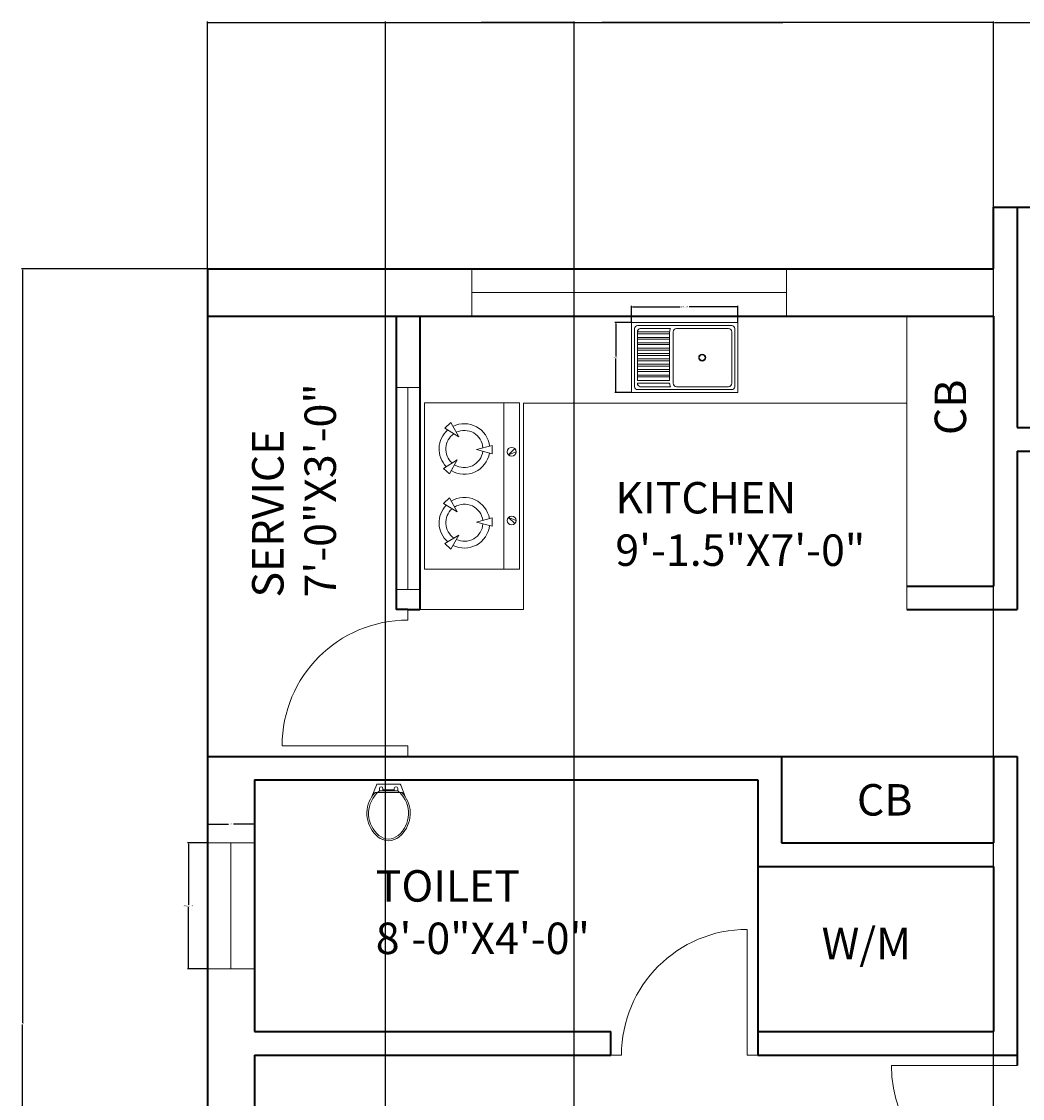
# Model space of a CAD drawing. Units: inches. Extents: x -59 to 444, y -680 to 63.
# Tile 5 of 9: x -59 to 132, y -143 to 63. Entities that reach past the tile are written whole.
import ezdxf

# ---------------------------------------------------------------- set-up
doc = ezdxf.new("R2010")
doc.units = ezdxf.units.IN
doc.header["$MEASUREMENT"] = 0
for name, color, linetype, lineweight in [('A-ANNO-DIMS', 2, 'Continuous', 18), ('A-ANNO-TEXT', 7, 'Continuous', 18), ('A-AREA-IDEN', 7, 'Continuous', 18), ('A-DOOR', 3, 'Continuous', 18), ('A-EQPM', 9, 'Continuous', 18), ('A-FLOR-CASE', 8, 'Continuous', 18), ('A-FLOR-FIXT', 9, 'Continuous', 18), ('A-GLAZ', 4, 'Continuous', 18), ('A-WALL', 7, 'Continuous', 35)]:
    doc.layers.add(name, color=color, linetype=linetype, lineweight=lineweight)
doc.styles.get("Standard").update_dxf_attribs({"font": 'arial.ttf'})
doc.dimstyles.get("Standard").update_dxf_attribs({"dimtxt": 0.18, "dimasz": 0.18, "dimexe": 0.18, "dimexo": 0.0625, "dimgap": 0.09, "dimtad": 0, "dimtih": 1, "dimtoh": 1, "dimdec": 0, "dimzin": 0, "dimdsep": 46, "dimlunit": 3, "dimtxsty": 'Standard', "dimcen": 0.09, "dimadec": 0, "dimazin": 0, "dimtfac": 1, "dimtdec": 0, "dimtofl": 0, "dimtmove": 0, "dimatfit": 3, "dimfxl": 1, "dimtolj": 1, "dimtzin": 0, "dimarcsym": 0})

# ---------------------------------------------------------------- blocks, each defined once
blk = doc.blocks.new('М12 540х820')
for p, q in [((0, 540), (-820, 540)), ((-820, 540), (-820, 0)), ((-45, 517.5), (-775, 517.5)), ((0, 0), (0, 540)), ((-797.5, 495), (-797.5, 45)), ((-775, 468), (-775, 72)), ((-347.5, 495), (-748, 495)), ((-320.5, 468), (-320.5, 72)), ((-301.7, 495), (-64.8, 495)), ((-293.7, 468), (-293.7, 472.5)), ((-293.7, 468), (-45, 468)), ((-293.7, 446.6), (-45, 446.6)), ((-293.7, 419.6), (-293.7, 446.6)), ((-293.7, 419.6), (-45, 419.6)), ((-45, 469.5), (-45, 468)), ((-45, 419.6), (-45, 446.6)), ((-22.5, 45), (-22.5, 495)), ((-293.7, 405), (-45, 405)), ((-293.7, 378), (-293.7, 405)), ((-293.7, 378), (-45, 378)), ((-293.7, 336.4), (-293.7, 363.4)), ((-293.7, 363.4), (-45, 363.4)), ((-293.7, 336.4), (-45, 336.4)), ((-45, 378), (-45, 405)), ((-45, 336.4), (-45, 363.4)), ((-293.7, 294.7), (-293.7, 321.7)), ((-293.7, 321.7), (-45, 321.7)), ((-293.7, 294.7), (-45, 294.7)), ((-293.7, 253.1), (-293.7, 280.1)), ((-293.7, 280.1), (-45, 280.1)), ((-293.7, 253.1), (-45, 253.1)), ((-45, 294.7), (-45, 321.7)), ((-45, 253.1), (-45, 280.1)), ((-293.7, 211.5), (-293.7, 238.5)), ((-293.7, 238.5), (-45, 238.5)), ((-293.7, 211.5), (-45, 211.5)), ((-293.7, 169.9), (-293.7, 196.9)), ((-293.7, 196.9), (-45, 196.9)), ((-293.7, 169.9), (-45, 169.9)), ((-45, 211.5), (-45, 238.5)), ((-45, 169.9), (-45, 196.9)), ((-293.7, 128.2), (-293.7, 155.2)), ((-293.7, 155.2), (-45, 155.2)), ((-293.7, 128.2), (-45, 128.2)), ((-293.7, 113.6), (-45, 113.6)), ((-293.7, 86.6), (-293.7, 113.6)), ((-293.7, 86.6), (-45, 86.6)), ((-45, 128.2), (-45, 155.2)), ((-45, 86.6), (-45, 113.6)), ((-820, 0), (0, 0)), ((-775, 22.5), (-45, 22.5)), ((-748, 45), (-347.5, 45)), ((-301.7, 45), (-64.8, 45)), ((-293.7, 72), (-45, 72)), ((-45, 70.5), (-45, 72))]:
    blk.add_line(p, q)
at = {"ltscale": 0.06}
for p, q in [((-820, 0), (-820, 540)), ((-820, 540), (0, 540)), ((0, 540), (0, 536.9)), ((0, 536.9), (0, 0)), ((-293.7, 446.6), (-45, 446.6)), ((-293.7, 405), (-293.7, 446.6)), ((-45, 446.6), (-45, 419.6)), ((-45, 419.6), (-45, 378)), ((-293.7, 363.4), (-293.7, 405)), ((-293.7, 321.7), (-293.7, 363.4)), ((-45, 378), (-45, 336.4)), ((-45, 336.4), (-45, 294.7)), ((-293.7, 280.1), (-293.7, 321.7)), ((-293.7, 238.5), (-293.7, 280.1)), ((-45, 294.7), (-45, 253.1)), ((-45, 253.1), (-45, 211.5)), ((-293.7, 196.9), (-293.7, 238.5)), ((-293.7, 155.2), (-293.7, 196.9)), ((-45, 211.5), (-45, 169.9)), ((-45, 169.9), (-45, 128.2)), ((-293.7, 113.6), (-293.7, 155.2)), ((-293.7, 72), (-293.7, 113.6)), ((-45, 128.2), (-45, 86.6)), ((-45, 86.6), (-45, 72)), ((0, 0), (-820, 0)), ((-45, 72), (-293.7, 72))]:
    blk.add_line(p, q, dxfattribs=at)
at = {"extrusion": (0, 0, -1)}
for centre, major_axis, start_param, end_param in [((-775, 495), (-15.9, 15.9), -0.785398, 0.785398), ((-775, 495), (-15.9, 15.9), -0.785398, 0.785398), ((-45, 495), (-15.9, -15.9), 2.356194, 3.926991), ((-45, 495), (-15.9, -15.9), 2.356194, 3.926991), ((-748, 468), (-19.1, -19.1), 0.785398, 2.356194), ((-748, 468), (-19.1, -19.1), 0.785398, 2.356194), ((-347.5, 468), (-19.1, 19.1), 0.785398, 2.356194), ((-347.5, 468), (-19.1, 19.1), 0.785398, 2.356194), ((-343.2, 468), (-35, 35), 1.779263, 2.356194), ((-343.2, 468), (-35, 35), 1.779263, 2.356192), ((-343.2, 468), (-35, 35), 2.356192, 2.356194), ((-72.3, 468.8), (-19.3, 19.3), 1.0328, 2.38382), ((-72.3, 468.8), (-19.3, 19.3), 1.0328, 1.064673), ((-72.3, 468.8), (-19.3, 19.3), 1.064673, 2.328569), ((-72.3, 468.8), (-19.3, 19.3), 2.328569, 2.38382), ((-545.5, 270), (-19.1, -19.1), 3.926991, 10.210176), ((-545.5, 270), (-19.1, -19.1), 3.926991, 10.210176), ((-545.5, 270), (-15.9, -15.9), 3.926991, 10.210176), ((-545.5, 270), (-15.9, -15.9), 3.926991, 10.210176), ((-775, 45), (-15.9, -15.9), 5.497787, 7.068583), ((-775, 45), (-15.9, -15.9), 5.497787, 7.068583), ((-748, 72), (-19.1, 19.1), 3.926991, 5.497787), ((-748, 72), (-19.1, 19.1), 3.926991, 5.497787), ((-347.5, 72), (-19.1, -19.1), 3.926991, 5.497787), ((-347.5, 72), (-19.1, -19.1), 3.926991, 5.497787), ((-343.2, 72), (-35, -35), 3.926991, 4.503922), ((-343.2, 72), (-35, -35), 3.926991, 4.503922), ((-72.3, 71.2), (-19.3, -19.3), 3.899365, 5.250385), ((-72.3, 71.2), (-19.3, -19.3), 5.218512, 5.250385), ((-72.3, 71.2), (-19.3, -19.3), 3.954617, 5.218512), ((-72.3, 71.2), (-19.3, -19.3), 3.899365, 3.954617), ((-45, 45), (-15.9, 15.9), 2.356194, 3.926991), ((-45, 45), (-15.9, 15.9), 2.356194, 3.926991)]:
    blk.add_ellipse(centre, major_axis=major_axis, ratio=1, start_param=start_param, end_param=end_param, dxfattribs=at)
blk = doc.blocks.new('WC-COMPACT')
for p, q in [((1.55, 9.19), (2, 9.19)), ((2, 9.19), (4.13, 9.19)), ((6.26, 9.19), (4.13, 9.19)), ((6.26, 9.19), (6.72, 9.19))]:
    blk.add_line(p, q)
for points in [[(4.13, 10.83), (2.07, 10.83, 0.31031), (1.81, 10.65), (0.96, 8.45, 0.209071)], [(2.38, 9.52), (2.38, 9.97, -1), (3.07, 9.97), (3.07, 9.73)], [(4.13, 10.83), (6.2, 10.83, -0.31031), (6.46, 10.65), (7.3, 8.45, -0.209071)], [(5.89, 9.52), (5.89, 9.97, 1), (5.2, 9.97), (5.2, 9.73)], [(0.96, 8.45, 0.383919), (2.1, 0.78, 0.163732), (4.13, 0, 0.359733)], [(1.79, 8.97, 0.431639), (2.3, 1.03, 0.162618), (4.13, 0.32, 0.470877)], [(1.55, 9.19, 0.040937), (0.96, 8.45, 0.163732)], [(2, 9.19, 0.014165), (1.79, 8.97, 0.162618)], [(2.38, 9.52, 0.022712), (2, 9.19, 0.162618)], [(4.13, 9.52), (2.38, 9.52, 0.022712)], [(4.13, 9.52), (5.89, 9.52, -0.476108)], [(6.26, 9.19, -0.448546), (5.96, 1.03, -0.162618), (4.13, 0.32, -0.470877)], [(7.3, 8.45, -0.383919), (6.17, 0.78, -0.163732), (4.13, 0, -0.359733)], [(5.89, 9.52, -0.022712), (6.26, 9.19, -0.162618)], [(6.72, 9.19, -0.040937), (7.3, 8.45, -0.163732)]]:
    blk.add_lwpolyline(points, format="xyb")
for points in [[(5.2, 9.73), (3.07, 9.73)], [(3.07, 9.73), (3.07, 9.52)], [(5.2, 9.73), (5.2, 9.52)]]:
    blk.add_lwpolyline(points)
blk = doc.blocks.new('WIN-60-W9')
for p, q in [((60, 9), (0, 9)), ((0, 9), (0, 0)), ((60, 0), (60, 9)), ((0, 4.5), (60, 4.5)), ((0, 0), (60, 0))]:
    blk.add_line(p, q)
blk = doc.blocks.new('WIN-24-W9')
for p, q in [((0, 24), (0, 0)), ((9, 24), (0, 24)), ((4.5, 24), (4.5, 0)), ((9, 0), (9, 24)), ((0, 0), (9, 0))]:
    blk.add_line(p, q)
blk = doc.blocks.new('WIN-SERVICE')
for p, q in [((0, 38.53), (0, 0)), ((4.5, 38.53), (0, 38.53)), ((2.25, 38.53), (2.25, 0)), ((4.5, 38.53), (4.5, 0)), ((0, 0), (4.5, 0))]:
    blk.add_line(p, q)
blk = doc.blocks.new('DOOR-SWING-24')
blk.add_line((24, 0), (0, 0))
blk.add_arc((24, 0), 24, 90, 180)
blk = doc.blocks.new('*D22')
at = {"layer": 'A-ANNO-DIMS', "color": 0, "lineweight": -2, "transparency": 16777216}
for p, q in [((-23.33, -93.94), (-27.05, -93.94)), ((-26.87, -94.12), (-26.87, -105.75)), ((-26.87, -117.76), (-26.87, -106.12)), ((-23.33, -117.94), (-27.05, -117.94))]:
    blk.add_line(p, q, dxfattribs=at)
at = {"layer": 'A-ANNO-DIMS', "color": 0, "transparency": 16777216}
for points in [[(-26.9, -94.12), (-26.84, -94.12), (-26.87, -93.94)], [(-26.9, -117.76), (-26.84, -117.76), (-26.87, -117.94)]]:
    blk.add_solid(points, dxfattribs=at)
at = {"layer": 'Defpoints', "color": 0, "transparency": 16777216}
for p in [(-23.27, -93.94), (-26.87, -117.94), (-23.27, -117.94)]:
    blk.add_point(p, dxfattribs=at)
at = {"layer": 'A-ANNO-DIMS', "color": 0, "transparency": 16777216, "insert": (-26.87, -105.94), "char_height": 0.18, "attachment_point": 5}
blk.add_mtext('\\A1;WINDOW 24 TYP.', dxfattribs=at)
blk = doc.blocks.new('*D23')
at = {"layer": 'A-ANNO-DIMS', "color": 0, "lineweight": -2, "transparency": 16777216}
for p, q in [((-23.27, -93.87), (-23.27, -90.16)), ((-23.09, -90.34), (-19.23, -90.34)), ((-14.45, -90.34), (-18.31, -90.34)), ((-14.27, -93.87), (-14.27, -90.16))]:
    blk.add_line(p, q, dxfattribs=at)
at = {"layer": 'A-ANNO-DIMS', "color": 0, "transparency": 16777216}
for points in [[(-23.09, -90.31), (-23.09, -90.37), (-23.27, -90.34)], [(-14.45, -90.31), (-14.45, -90.37), (-14.27, -90.34)]]:
    blk.add_solid(points, dxfattribs=at)
at = {"layer": 'Defpoints', "color": 0, "transparency": 16777216}
for p in [(-23.27, -90.34), (-23.27, -93.94), (-14.27, -93.94)]:
    blk.add_point(p, dxfattribs=at)
at = {"layer": 'A-ANNO-DIMS', "color": 0, "transparency": 16777216, "insert": (-18.77, -90.34), "char_height": 0.18, "attachment_point": 5}
blk.add_mtext('\\A1;9 TYP.', dxfattribs=at)
blk = doc.blocks.new('*D28')
at = {"layer": 'A-ANNO-DIMS', "color": 0, "lineweight": -2, "transparency": 16777216}
for p, q in [((57.67, 5.36), (57.67, 8.51)), ((57.85, 8.33), (66.93, 8.33)), ((77.72, 8.33), (68.64, 8.33)), ((77.9, 5.36), (77.9, 8.51))]:
    blk.add_line(p, q, dxfattribs=at)
at = {"layer": 'A-ANNO-DIMS', "color": 0, "transparency": 16777216}
for points in [[(57.85, 8.36), (57.85, 8.3), (57.67, 8.33)], [(77.72, 8.36), (77.72, 8.3), (77.9, 8.33)]]:
    blk.add_solid(points, dxfattribs=at)
at = {"layer": 'Defpoints', "color": 0, "transparency": 16777216}
for p in [(57.67, 8.33), (57.67, 5.3), (77.9, 5.3)]:
    blk.add_point(p, dxfattribs=at)
at = {"layer": 'A-ANNO-DIMS', "color": 0, "transparency": 16777216, "insert": (67.79, 8.33), "char_height": 0.18, "attachment_point": 5}
blk.add_mtext('\\A1;SINK 20 TYP.', dxfattribs=at)
blk = doc.blocks.new('*D29')
at = {"layer": 'A-ANNO-DIMS', "color": 0, "lineweight": -2, "transparency": 16777216}
for p, q in [((57.61, 5.3), (54.46, 5.3)), ((54.64, 5.12), (54.64, -1.18)), ((54.64, -7.84), (54.64, -1.54)), ((57.61, -8.02), (54.46, -8.02))]:
    blk.add_line(p, q, dxfattribs=at)
at = {"layer": 'A-ANNO-DIMS', "color": 0, "transparency": 16777216}
for points in [[(54.61, 5.12), (54.67, 5.12), (54.64, 5.3)], [(54.61, -7.84), (54.67, -7.84), (54.64, -8.02)]]:
    blk.add_solid(points, dxfattribs=at)
at = {"layer": 'Defpoints', "color": 0, "transparency": 16777216}
for p in [(57.67, 5.3), (54.64, -8.02), (57.67, -8.02)]:
    blk.add_point(p, dxfattribs=at)
at = {"layer": 'A-ANNO-DIMS', "color": 0, "transparency": 16777216, "insert": (54.64, -1.36), "char_height": 0.18, "attachment_point": 5}
blk.add_mtext('\\A1;13 TYP.', dxfattribs=at)
blk = doc.blocks.new('*D48')
at = {"layer": 'A-ANNO-DIMS', "color": 0, "lineweight": -2, "transparency": 16777216}
for p, q in [((-23.33, 15.56), (-58.7, 15.56)), ((-58.52, 15.38), (-58.52, -128.25)), ((-58.52, -272.26), (-58.52, -128.62)), ((-23.33, -272.44), (-58.7, -272.44))]:
    blk.add_line(p, q, dxfattribs=at)
at = {"layer": 'A-ANNO-DIMS', "color": 0, "transparency": 16777216}
for points in [[(-58.55, 15.38), (-58.49, 15.38), (-58.52, 15.56)], [(-58.55, -272.26), (-58.49, -272.26), (-58.52, -272.44)]]:
    blk.add_solid(points, dxfattribs=at)
at = {"layer": 'Defpoints', "color": 0, "transparency": 16777216}
for p in [(-23.27, 15.56), (-58.52, -272.44), (-23.27, -272.44)]:
    blk.add_point(p, dxfattribs=at)
at = {"layer": 'A-ANNO-DIMS', "color": 0, "transparency": 16777216, "insert": (-58.52, -128.44), "char_height": 0.18, "attachment_point": 5}
blk.add_mtext('\\A1;288', dxfattribs=at)
blk = doc.blocks.new('*D51')
at = {"layer": 'A-ANNO-DIMS', "color": 0, "lineweight": -2, "transparency": 16777216}
for p, q in [((-23.27, 15.63), (-23.27, 62.74)), ((-23.09, 62.56), (51.45, 62.56)), ((126.55, 62.56), (52.01, 62.56)), ((126.73, 27.38), (126.73, 62.74))]:
    blk.add_line(p, q, dxfattribs=at)
at = {"layer": 'A-ANNO-DIMS', "color": 0, "transparency": 16777216}
for points in [[(-23.09, 62.59), (-23.09, 62.53), (-23.27, 62.56)], [(126.55, 62.59), (126.55, 62.53), (126.73, 62.56)]]:
    blk.add_solid(points, dxfattribs=at)
at = {"layer": 'Defpoints', "color": 0, "transparency": 16777216}
for p in [(126.73, 62.56), (126.73, 27.31), (-23.27, 15.56)]:
    blk.add_point(p, dxfattribs=at)
at = {"layer": 'A-ANNO-DIMS', "color": 0, "transparency": 16777216, "insert": (51.73, 62.56), "char_height": 0.18, "attachment_point": 5}
blk.add_mtext('\\A1;150', dxfattribs=at)
blk = doc.blocks.new('*D52')
at = {"layer": 'A-ANNO-DIMS', "color": 0, "lineweight": -2, "transparency": 16777216}
for p, q in [((126.73, 27.38), (126.73, 62.74)), ((126.91, 62.56), (196.97, 62.56)), ((267.55, 62.56), (197.49, 62.56)), ((267.73, 27.38), (267.73, 62.74))]:
    blk.add_line(p, q, dxfattribs=at)
at = {"layer": 'A-ANNO-DIMS', "color": 0, "transparency": 16777216}
for points in [[(126.91, 62.59), (126.91, 62.53), (126.73, 62.56)], [(267.55, 62.59), (267.55, 62.53), (267.73, 62.56)]]:
    blk.add_solid(points, dxfattribs=at)
at = {"layer": 'Defpoints', "color": 0, "transparency": 16777216}
for p in [(267.73, 62.56), (126.73, 27.31), (267.73, 27.31)]:
    blk.add_point(p, dxfattribs=at)
at = {"layer": 'A-ANNO-DIMS', "color": 0, "transparency": 16777216, "insert": (197.23, 62.56), "char_height": 0.18, "attachment_point": 5}
blk.add_mtext('\\A1;141', dxfattribs=at)
blk = doc.blocks.new('*D54')
at = {"layer": 'A-ANNO-DIMS', "color": 0, "lineweight": -2, "transparency": 16777216}
for p, q in [((10.73, -344.37), (10.73, 62.74)), ((10.91, 62.56), (28.51, 62.56)), ((46.55, 62.56), (28.95, 62.56)), ((46.73, -344.37), (46.73, 62.74))]:
    blk.add_line(p, q, dxfattribs=at)
at = {"layer": 'A-ANNO-DIMS', "color": 0, "transparency": 16777216}
for points in [[(10.91, 62.59), (10.91, 62.53), (10.73, 62.56)], [(46.55, 62.59), (46.55, 62.53), (46.73, 62.56)]]:
    blk.add_solid(points, dxfattribs=at)
at = {"layer": 'Defpoints', "color": 0, "transparency": 16777216}
for p in [(46.73, 62.56), (10.73, -344.44), (46.73, -344.44)]:
    blk.add_point(p, dxfattribs=at)
at = {"layer": 'A-ANNO-DIMS', "color": 0, "transparency": 16777216, "insert": (28.73, 62.56), "char_height": 0.18, "attachment_point": 5}
blk.add_mtext('\\A1;36', dxfattribs=at)
blk = doc.blocks.new('*D55')
at = {"layer": 'A-ANNO-DIMS', "color": 0, "lineweight": -2, "transparency": 16777216}
for p, q in [((46.73, -344.37), (46.73, 62.74)), ((46.91, 62.56), (86.51, 62.56)), ((126.55, 62.56), (86.95, 62.56)), ((126.73, -344.37), (126.73, 62.74))]:
    blk.add_line(p, q, dxfattribs=at)
at = {"layer": 'A-ANNO-DIMS', "color": 0, "transparency": 16777216}
for points in [[(46.91, 62.59), (46.91, 62.53), (46.73, 62.56)], [(126.55, 62.59), (126.55, 62.53), (126.73, 62.56)]]:
    blk.add_solid(points, dxfattribs=at)
at = {"layer": 'Defpoints', "color": 0, "transparency": 16777216}
for p in [(126.73, 62.56), (46.73, -344.44), (126.73, -344.44)]:
    blk.add_point(p, dxfattribs=at)
at = {"layer": 'A-ANNO-DIMS', "color": 0, "transparency": 16777216, "insert": (86.73, 62.56), "char_height": 0.18, "attachment_point": 5}
blk.add_mtext('\\A1;80', dxfattribs=at)
blk = doc.blocks.new('*D56')
at = {"layer": 'A-ANNO-DIMS', "color": 0, "lineweight": -2, "transparency": 16777216}
for p, q in [((126.73, -344.37), (126.73, 62.74)), ((126.91, 62.56), (158.65, 62.56)), ((191.05, 62.56), (159.3, 62.56)), ((191.23, -344.37), (191.23, 62.74))]:
    blk.add_line(p, q, dxfattribs=at)
at = {"layer": 'A-ANNO-DIMS', "color": 0, "transparency": 16777216}
for points in [[(126.91, 62.59), (126.91, 62.53), (126.73, 62.56)], [(191.05, 62.59), (191.05, 62.53), (191.23, 62.56)]]:
    blk.add_solid(points, dxfattribs=at)
at = {"layer": 'Defpoints', "color": 0, "transparency": 16777216}
for p in [(191.23, 62.56), (126.73, -344.44), (191.23, -344.44)]:
    blk.add_point(p, dxfattribs=at)
at = {"layer": 'A-ANNO-DIMS', "color": 0, "transparency": 16777216, "insert": (158.98, 62.56), "char_height": 0.18, "attachment_point": 5}
blk.add_mtext('\\A1;64.5', dxfattribs=at)

msp = doc.modelspace()

# ---------------------------------------------------------------- linework, layer by layer
at = {"layer": 'A-DOOR'}
for p, q in [((14.98, -51.44), (14.98, -49.44)), ((14.98, -77.44), (14.98, -75.44)), ((55.73, -134.44), (53.73, -134.44)), ((81.73, -134.44), (79.73, -134.44)), ((131.23, -136.44), (107.23, -136.44))]:
    msp.add_line(p, q, dxfattribs=at)
msp.add_arc((131.75, -136.44), 24.52, 180, 258.1877, dxfattribs=at)
at = {"layer": 'A-EQPM'}
for p, q in [((33.31, -10.02), (33.31, -41.73)), ((22.06, -14.85), (23.18, -13.75)), ((23.18, -13.75), (24.68, -16.45)), ((24.68, -16.45), (22.06, -14.85)), ((28.05, -18.89), (31.03, -18.15)), ((31.03, -18.15), (31.03, -19.71)), ((31.03, -19.71), (28.05, -18.89)), ((21.77, -22.49), (24.4, -20.86)), ((22.92, -23.56), (21.77, -22.49)), ((24.4, -20.86), (22.92, -23.56)), ((22.92, -28.12), (21.77, -29.18)), ((24.4, -30.81), (22.92, -28.12)), ((21.77, -29.18), (24.4, -30.81)), ((31.03, -31.96), (28.05, -32.78)), ((28.05, -32.78), (31.03, -33.53)), ((31.03, -33.53), (31.03, -31.96)), ((24.68, -35.22), (22.06, -36.82)), ((22.06, -36.82), (23.18, -37.92)), ((23.18, -37.92), (24.68, -35.22))]:
    msp.add_line(p, q, dxfattribs=at)
at = {"layer": 'A-EQPM', "ltscale": 20}
for p, q in [((34.2, -19.92), (35.37, -18.73)), ((35.62, -19.32), (34.2, -19.92)), ((34.2, -31.84), (35.37, -33.02)), ((35.62, -32.43), (34.2, -31.84))]:
    msp.add_line(p, q, dxfattribs=at)
at = {"layer": 'A-EQPM'}
msp.add_lwpolyline([(18.13, -41.73), (18.13, -10.02), (36.25, -10.02), (36.25, -41.73)], close=True, dxfattribs=at)
at = {"layer": 'A-EQPM', "ltscale": 20}
for centre in [(34.78, -19.32), (34.78, -32.43)]:
    msp.add_circle(centre, 0.834, dxfattribs=at)
at = {"layer": 'A-EQPM'}
for centre, radius, start, end in [((25.76, -18.8), 4.83, 6.4005, 116.769), ((25.76, -18.8), 4.83, 131.2225, 224.1627), ((25.76, -18.8), 3.54, 124.5561, 228.8027), ((25.76, -18.8), 3.54, 3.5753, 115.9207), ((25.76, -18.8), 4.83, 238.853, 350.7562), ((25.76, -18.8), 3.54, 237.9778, 353.02), ((25.76, -32.87), 4.83, 9.2438, 121.147), ((25.76, -32.87), 4.83, 135.8373, 228.7775), ((25.76, -32.87), 3.54, 131.1973, 235.4439), ((25.76, -32.87), 3.54, 6.98, 122.0222), ((25.76, -32.87), 4.83, 243.231, 353.5995), ((25.76, -32.87), 3.54, 244.0793, 356.4247)]:
    msp.add_arc(centre, radius, start, end, dxfattribs=at)
at = {"layer": 'A-FLOR-CASE'}
for p, q in [((110.14, -49.44), (110.14, 6.56)), ((37.06, -49.44), (37.06, -10.04)), ((37.06, -10.04), (110.14, -10.04)), ((17.23, -49.44), (37.06, -49.44))]:
    msp.add_line(p, q, dxfattribs=at)
at = {"layer": 'A-WALL'}
for p, q in [((126.73, 15.56), (126.73, 27.31)), ((126.73, 27.31), (131.23, 27.31)), ((131.23, 27.31), (131.23, -14.69)), ((131.23, 27.31), (263.23, 27.31)), ((-23.27, 15.56), (126.73, 15.56)), ((-23.27, 15.56), (-23.27, -272.44)), ((-23.27, 6.56), (126.73, 6.56)), ((12.73, 6.56), (12.73, -49.44)), ((17.23, 6.56), (17.23, -49.44)), ((126.73, 6.56), (126.73, -44.94)), ((131.23, -14.69), (173.23, -14.69)), ((131.23, -19.19), (173.23, -19.19)), ((131.23, -19.19), (131.23, -49.44)), ((110.14, -44.94), (126.73, -44.94)), ((14.98, -49.44), (12.73, -49.44)), ((14.98, -49.44), (17.23, -49.44)), ((110.14, -49.44), (131.23, -49.44)), ((-23.27, -77.44), (131.23, -77.44)), ((12.73, -77.44), (17.23, -77.44)), ((86.23, -77.44), (86.23, -93.94)), ((126.73, -77.44), (126.73, -93.94)), ((131.23, -77.44), (131.23, -136.44)), ((-14.27, -81.94), (81.73, -81.94)), ((-14.27, -81.94), (-14.27, -129.94)), ((81.73, -81.94), (81.73, -134.44)), ((86.23, -93.94), (126.73, -93.94)), ((81.73, -98.44), (126.73, -98.44)), ((126.73, -98.44), (126.73, -129.94)), ((-14.27, -129.94), (53.73, -129.94)), ((53.73, -134.44), (53.73, -129.94)), ((81.73, -129.94), (126.73, -129.94)), ((-14.27, -134.44), (53.73, -134.44)), ((-14.27, -134.44), (-14.27, -263.44)), ((81.73, -134.44), (131.23, -134.44))]:
    msp.add_line(p, q, dxfattribs=at)

# ---------------------------------------------------------------- block references
at = {"layer": 'A-DOOR'}
msp.add_blockref('DOOR-SWING-24', (-9.02, -75.44), dxfattribs=at)
at = {"layer": 'A-DOOR', "extrusion": (0, 0, -1), "zscale": -1, "rotation": 270}
msp.add_blockref('DOOR-SWING-24', (-79.73, -110.44), dxfattribs=at)
at = {"layer": 'A-FLOR-FIXT', "xscale": 0.0246684035300764, "yscale": 0.0246684035300764, "zscale": 0.0246684035300764, "rotation": 180}
msp.add_blockref('М12 540х820', (57.67, 5.3), dxfattribs=at)
at = {"layer": 'A-FLOR-FIXT'}
msp.add_blockref('WC-COMPACT', (7.16, -93.55), dxfattribs=at)
at = {"layer": 'A-GLAZ'}
for name, p in [('WIN-60-W9', (27.19, 6.56)), ('WIN-SERVICE', (12.73, -45.59))]:
    msp.add_blockref(name, p, dxfattribs=at)
at = {"layer": 'A-GLAZ', "rotation": 180}
msp.add_blockref('WIN-24-W9', (-14.27, -93.94), dxfattribs=at)

# ---------------------------------------------------------------- texts
at = {"layer": 'A-ANNO-TEXT', "insert": (115.48, -16.14), "char_height": 6, "attachment_point": 1, "rotation": 90}
msp.add_mtext('CB', dxfattribs=at)
at = {"layer": 'A-ANNO-TEXT', "char_height": 6, "attachment_point": 1}
for s, insert in [('CB', (100.65, -82.73)), ('W/M', (93.92, -110.14))]:
    msp.add_mtext(s, dxfattribs=dict(at, insert=insert))
at = {"layer": 'A-AREA-IDEN', "insert": (-14.74, -47.13), "char_height": 6, "attachment_point": 1, "rotation": 90}
msp.add_mtext('SERVICE\\P7\'-0"X3\'-0"', dxfattribs=at)
at = {"layer": 'A-AREA-IDEN', "char_height": 6, "attachment_point": 1}
for s, insert in [('KITCHEN\\P9\'-1.5"X7\'-0"', (54.56, -25.1)), ('TOILET\\P8\'-0"X4\'-0"', (8.85, -99.15))]:
    msp.add_mtext(s, dxfattribs=dict(at, insert=insert))

# ---------------------------------------------------------------- dimensions: what is measured, and where the dimension line sits
at = {"layer": 'A-ANNO-DIMS'}
for base, p1, p2, override, picture, middle in [((126.73, 62.56), (-23.27, 15.56), (126.73, 27.31), {"dimdec": 0, "dimlfac": 1, "dimrnd": 0, "dimzin": 0, "dimdsep": 46, "dimlunit": 2}, '*D51', (51.73, 62.56)), ((46.73, 62.56), (10.73, -344.44), (46.73, -344.44), {"dimdec": 0, "dimlfac": 1, "dimrnd": 0, "dimzin": 0, "dimdsep": 46, "dimlunit": 2}, '*D54', (28.73, 62.56)), ((126.73, 62.56), (46.73, -344.44), (126.73, -344.44), {"dimdec": 0, "dimlfac": 1, "dimrnd": 0, "dimzin": 0, "dimdsep": 46, "dimlunit": 2}, '*D55', (86.73, 62.56)), ((267.73, 62.56), (126.73, 27.31), (267.73, 27.31), {"dimdec": 0, "dimlfac": 1, "dimrnd": 0, "dimzin": 0, "dimdsep": 46, "dimlunit": 2}, '*D52', (197.23, 62.56)), ((191.23, 62.56), (126.73, -344.44), (191.23, -344.44), {"dimdec": 1, "dimlfac": 1, "dimrnd": 0, "dimzin": 0, "dimdsep": 46, "dimlunit": 2}, '*D56', (158.98, 62.56))]:
    dim = msp.add_linear_dim(base=base, p1=p1, p2=p2, dimstyle='Standard', override=override, dxfattribs=at)
    dim.commit()
    dim.dimension.update_dxf_attribs({"geometry": picture, "text_midpoint": middle})
dim = msp.add_linear_dim(base=(-58.52, -272.44), p1=(-23.27, 15.56), p2=(-23.27, -272.44), angle=90, dimstyle='Standard', override={"dimdec": 0, "dimlfac": 1, "dimrnd": 0, "dimzin": 0, "dimdsep": 46, "dimlunit": 2}, dxfattribs=at)
dim.commit()
dim.dimension.update_dxf_attribs({"geometry": '*D48', "text_midpoint": (-58.52, -128.44)})
for base, p1, p2, angle, text, picture, middle in [((57.67, 8.33), (77.9, 5.3), (57.67, 5.3), 180, 'SINK <> TYP.', '*D28', (67.79, 8.33)), ((54.64, -8.02), (57.67, 5.3), (57.67, -8.02), 270, '<> TYP.', '*D29', (54.64, -1.36)), ((-23.27, -90.34), (-14.27, -93.94), (-23.27, -93.94), 180, '<> TYP.', '*D23', (-18.77, -90.34)), ((-26.87, -117.94), (-23.27, -93.94), (-23.27, -117.94), 270, 'WINDOW <> TYP.', '*D22', (-26.87, -105.94))]:
    dim = msp.add_linear_dim(base=base, p1=p1, p2=p2, angle=angle, text=text, dimstyle='Standard', override={"dimdec": 0, "dimlfac": 1, "dimrnd": 0, "dimzin": 0, "dimdsep": 46, "dimlunit": 2}, dxfattribs=at)
    dim.commit()
    dim.dimension.update_dxf_attribs({"geometry": picture, "text_midpoint": middle})

doc.saveas('drawing.dxf')
